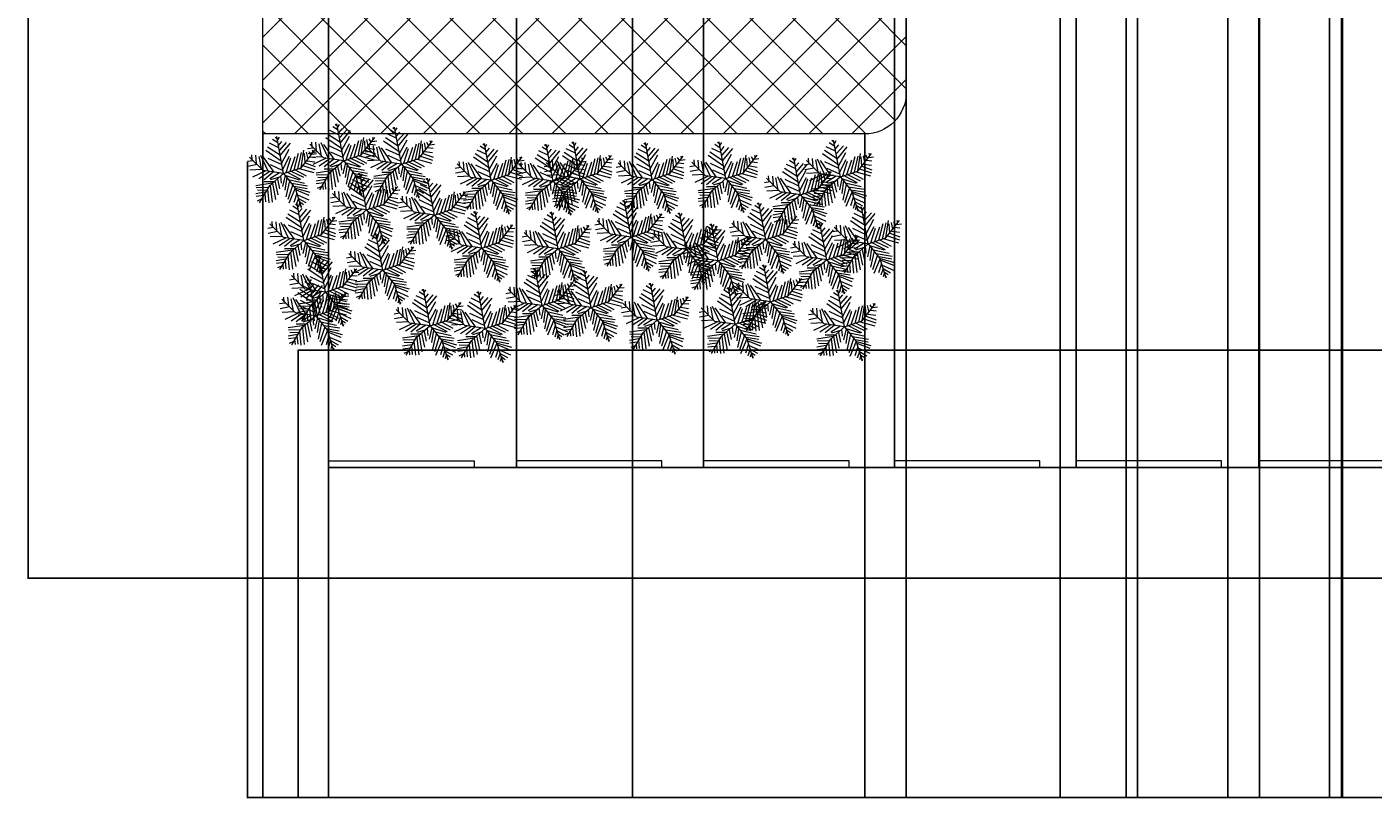
# Model space of a CAD drawing. Units: inches. Extents: x 818 to 1898, y 976 to 2364.
# Tile 1 of 96: x 818 to 1207, y 976 to 1198. Entities that reach past the tile are written whole.
import ezdxf

# ---------------------------------------------------------------- set-up
doc = ezdxf.new("R2010")
doc.units = ezdxf.units.IN
doc.header["$LTSCALE"] = 5
doc.header["$MEASUREMENT"] = 0
for name, color, linetype, lineweight in [('A-ANNO-DIMS', 2, 'Continuous', 18), ('C-PAVE-PATT', 8, 'Continuous', 9), ('C-ROAD', 8, 'Continuous', 25), ('C-ROAD-MRKG', 7, 'Continuous', 13), ('L-PAVE', 8, 'Continuous', 18)]:
    doc.layers.add(name, color=color, linetype=linetype, lineweight=lineweight)
doc.layers.add('L-PLNT', color=116, linetype='Continuous', lineweight=13, true_color=0x136734)
doc.styles.get("Standard").update_dxf_attribs({"font": 'arial.ttf'})
doc.dimstyles.get("Standard").update_dxf_attribs({"dimtxt": 0.18, "dimasz": 0.18, "dimexe": 0.18, "dimexo": 0.0625, "dimgap": 0.09, "dimtad": 0, "dimtih": 1, "dimtoh": 1, "dimdec": 4, "dimzin": 0, "dimdsep": 46, "dimtxsty": 'Standard', "dimcen": 0.09, "dimadec": 0, "dimazin": 0, "dimtfac": 1, "dimtdec": 4, "dimtofl": 0, "dimtmove": 0, "dimatfit": 3, "dimfxl": 1, "dimtolj": 1, "dimtzin": 0, "dimarcsym": 0})

# ---------------------------------------------------------------- blocks, each defined once
blk = doc.blocks.new('SHRUB-ACCENT')
for p, q in [((8.8, 18.63), (7.25, 19.67)), ((8.53, 19.84), (7.99, 20.28)), ((10.44, 9.82), (8.47, 20.47)), ((8.74, 19.5), (9.21, 20.28)), ((9.75, 13.42), (5.28, 16.46)), ((9.48, 15.07), (5.82, 17.41)), ((9.08, 17.24), (6.37, 18.54)), ((9.01, 17.93), (9.96, 19.06)), ((9.35, 16.54), (11.31, 18.8)), ((9.48, 14.98), (12.39, 18.54)), ((9.89, 12.9), (12.06, 16.89)), ((13.48, 10.9), (14.76, 15.68)), ((14.56, 11.16), (15.58, 15.85)), ((15.49, 11.5), (19.41, 16.55)), ((15.51, 11.51), (16.25, 16.54)), ((16.39, 15.59), (16.53, 12.9)), ((17, 15.94), (17.41, 14.03)), ((17.68, 16.2), (18.29, 15.16)), ((18.62, 15.42), (19.98, 15.59)), ((18.69, 16.63), (18.9, 15.94)), ((1.56, 13.51), (0, 13.25)), ((2.84, 12.38), (0.14, 11.86)), ((4.55, 10.66), (0.62, 14.58)), ((1.35, 13.77), (1.22, 15.24)), ((2.3, 15.16), (2.51, 12.72)), ((3.25, 14.72), (3.93, 11.25)), ((3.79, 15.07), (5.89, 10.55)), ((7.72, 10.21), (4.67, 14.55)), ((5.89, 14.29), (9.89, 12.38)), ((6.57, 12.38), (10.23, 10.73)), ((10.23, 11.07), (12.12, 14.81)), ((11.17, 10.12), (12.53, 14.37)), ((12.33, 10.47), (13.75, 14.72)), ((15.98, 12.12), (19.44, 10.99)), ((16.66, 12.9), (19.57, 11.86)), ((17.2, 13.51), (19.44, 13.16)), ((18.02, 14.63), (19.57, 14.46)), ((4.2, 10.99), (0.68, 10.81)), ((5.15, 10.47), (1.49, 8.73)), ((6.43, 10.38), (3.32, 8.3)), ((10.44, 9.82), (4.55, 10.66)), ((7.45, 10.21), (4.81, 8.04)), ((10.44, 9.82), (6.23, 6.17)), ((9.21, 10.03), (6.43, 8.3)), ((9.21, 8.73), (6.7, 7.95)), ((8.67, 8.21), (9.28, 5.43)), ((9.55, 9.16), (9.75, 7.08)), ((10.9, 9.25), (10.16, 6.04)), ((10.44, 9.82), (15.49, 11.5)), ((10.44, 9.82), (13.8, 5.61)), ((10.77, 9.34), (14.97, 8.04)), ((11.38, 8.64), (10.84, 5)), ((11.65, 10.12), (15.31, 8.21)), ((11.85, 8.12), (16.46, 7.08)), ((12.53, 10.47), (16.19, 8.73)), ((13.82, 10.9), (17, 9.16)), ((14.97, 11.25), (19.17, 10.12)), ((7.18, 6.99), (2.44, 6.3)), ((5.15, 4.39), (2.44, 3.95)), ((5.89, 5.78), (2.51, 5.69)), ((5.42, 4.91), (2.91, 5)), ((6.23, 6.17), (3.43, 1.4)), ((7.59, 7.43), (4.81, 7.43)), ((5.01, 4.04), (5.21, 1.61)), ((5.76, 5.34), (6.16, 1.35)), ((6.57, 6.39), (7.11, 1.52)), ((7.25, 6.99), (8.06, 2.31)), ((7.92, 7.69), (8.8, 3.69)), ((12.12, 7.69), (11.11, 3.09)), ((13.07, 6.65), (11.65, 2.31)), ((13.82, 5.6), (11.99, 1.26)), ((12.73, 6.99), (17.34, 6.3)), ((14.22, 4.13), (13.41, 1.44)), ((13.48, 6.13), (17.2, 5.52)), ((13.8, 5.61), (15.49, 0)), ((13.88, 5.6), (18.02, 4.39)), ((14.02, 5.08), (17.68, 3.61)), ((4.67, 3.43), (2.51, 3.17)), ((4, 2.39), (2.78, 1.87)), ((4.33, 2.91), (4.47, 1.52)), ((14.7, 2.74), (14.09, 0.74)), ((14.43, 3.69), (17.74, 2.22)), ((14.7, 2.65), (16.86, 1.44)), ((15.04, 1.26), (14.76, 0.31)), ((15.04, 1.7), (16.19, 0.92)), ((15.44, 0.48), (15.71, 0.31))]:
    blk.add_line(p, q)
blk = doc.blocks.new('LANE-STRIPE')
at = {"ltscale": 5}
for p, q in [((0, 2), (42, 2)), ((0, 2), (0, 0)), ((0, 0), (42, 0)), ((42, 2), (42, 0))]:
    blk.add_line(p, q, dxfattribs=at)
blk = doc.blocks.new('*D56')
at = {"layer": 'A-ANNO-DIMS', "color": 0, "lineweight": -2, "ltscale": 5, "transparency": 16777216}
for p, q in [((885.95, 1167.31), (885.95, 975.66)), ((1828.91, 1167.31), (1828.91, 975.66)), ((886.13, 975.84), (1357.14, 975.84)), ((1828.73, 975.84), (1357.72, 975.84))]:
    blk.add_line(p, q, dxfattribs=at)
at = {"layer": 'A-ANNO-DIMS', "color": 0, "ltscale": 5, "transparency": 16777216}
for points in [[(886.13, 975.87), (886.13, 975.81), (885.95, 975.84)], [(1828.73, 975.87), (1828.73, 975.81), (1828.91, 975.84)]]:
    blk.add_solid(points, dxfattribs=at)
at = {"layer": 'Defpoints', "color": 0, "ltscale": 5, "transparency": 16777216}
for p in [(885.95, 1167.37), (1828.91, 1167.37), (1828.91, 975.84)]:
    blk.add_point(p, dxfattribs=at)
at = {"layer": 'A-ANNO-DIMS', "color": 0, "ltscale": 5, "transparency": 16777216, "insert": (1357.43, 975.84), "char_height": 0.18, "attachment_point": 5}
blk.add_mtext('\\A1;943', dxfattribs=at)
blk = doc.blocks.new('*D58')
at = {"layer": 'A-ANNO-DIMS', "color": 0, "lineweight": -2, "ltscale": 5, "transparency": 16777216}
for p, q in [((881.51, 1159.31), (881.51, 975.66)), ((1834.44, 1145.13), (1834.44, 975.66)), ((881.69, 975.84), (1357.68, 975.84)), ((1834.26, 975.84), (1358.26, 975.84))]:
    blk.add_line(p, q, dxfattribs=at)
at = {"layer": 'A-ANNO-DIMS', "color": 0, "ltscale": 5, "transparency": 16777216}
for points in [[(881.69, 975.87), (881.69, 975.81), (881.51, 975.84)], [(1834.26, 975.87), (1834.26, 975.81), (1834.44, 975.84)]]:
    blk.add_solid(points, dxfattribs=at)
at = {"layer": 'Defpoints', "color": 0, "ltscale": 5, "transparency": 16777216}
for p in [(881.51, 1159.38), (1834.44, 1145.19), (1834.44, 975.84)]:
    blk.add_point(p, dxfattribs=at)
at = {"layer": 'A-ANNO-DIMS', "color": 0, "ltscale": 5, "transparency": 16777216, "insert": (1357.97, 975.84), "char_height": 0.18, "attachment_point": 5}
blk.add_mtext('\\A1;953', dxfattribs=at)
blk = doc.blocks.new('*D59')
at = {"layer": 'A-ANNO-DIMS', "color": 0, "lineweight": -2, "ltscale": 5, "transparency": 16777216}
for p, q in [((1251.64, 2300.39), (818.03, 2300.39)), ((818.21, 2300.21), (818.21, 1669.95)), ((818.21, 1039.32), (818.21, 1669.59)), ((896.05, 1039.14), (818.03, 1039.14))]:
    blk.add_line(p, q, dxfattribs=at)
at = {"layer": 'A-ANNO-DIMS', "color": 0, "ltscale": 5, "transparency": 16777216}
for points in [[(818.18, 2300.21), (818.24, 2300.21), (818.21, 2300.39)], [(818.18, 1039.32), (818.24, 1039.32), (818.21, 1039.14)]]:
    blk.add_solid(points, dxfattribs=at)
at = {"layer": 'Defpoints', "color": 0, "ltscale": 5, "transparency": 16777216}
for p in [(818.21, 2300.39), (1251.71, 2300.39), (896.11, 1039.14)]:
    blk.add_point(p, dxfattribs=at)
at = {"layer": 'A-ANNO-DIMS', "color": 0, "ltscale": 5, "transparency": 16777216, "insert": (818.21, 1669.77), "char_height": 0.18, "attachment_point": 5}
blk.add_mtext('\\A1;1261.2', dxfattribs=at)
blk = doc.blocks.new('*D62')
at = {"layer": 'A-ANNO-DIMS', "color": 0, "lineweight": -2, "ltscale": 5, "transparency": 16777216}
for p, q in [((1116.19, 1235.9), (1116.19, 975.66)), ((1406.73, 1235.9), (1406.73, 975.66)), ((1116.37, 975.84), (1260.99, 975.84)), ((1406.55, 975.84), (1261.92, 975.84))]:
    blk.add_line(p, q, dxfattribs=at)
at = {"layer": 'A-ANNO-DIMS', "color": 0, "ltscale": 5, "transparency": 16777216}
for points in [[(1116.37, 975.87), (1116.37, 975.81), (1116.19, 975.84)], [(1406.55, 975.87), (1406.55, 975.81), (1406.73, 975.84)]]:
    blk.add_solid(points, dxfattribs=at)
at = {"layer": 'Defpoints', "color": 0, "ltscale": 5, "transparency": 16777216}
for p in [(1116.19, 1235.96), (1406.73, 1235.96), (1406.73, 975.84)]:
    blk.add_point(p, dxfattribs=at)
at = {"layer": 'A-ANNO-DIMS', "color": 0, "ltscale": 5, "transparency": 16777216, "insert": (1261.46, 975.84), "char_height": 0.18, "attachment_point": 5}
blk.add_mtext('\\A1;290.54', dxfattribs=at)
blk = doc.blocks.new('*D77')
at = {"layer": 'A-ANNO-DIMS', "color": 0, "lineweight": -2, "ltscale": 5, "transparency": 16777216}
for p, q in [((992.73, 1202.9), (992.73, 975.66)), ((896.11, 1104.9), (896.11, 975.66)), ((896.29, 975.84), (944.04, 975.84)), ((992.55, 975.84), (944.8, 975.84))]:
    blk.add_line(p, q, dxfattribs=at)
at = {"layer": 'A-ANNO-DIMS', "color": 0, "ltscale": 5, "transparency": 16777216}
for points in [[(896.29, 975.87), (896.29, 975.81), (896.11, 975.84)], [(992.55, 975.87), (992.55, 975.81), (992.73, 975.84)]]:
    blk.add_solid(points, dxfattribs=at)
at = {"layer": 'Defpoints', "color": 0, "ltscale": 5, "transparency": 16777216}
for p in [(992.73, 1202.96), (896.11, 1104.97), (992.73, 975.84)]:
    blk.add_point(p, dxfattribs=at)
at = {"layer": 'A-ANNO-DIMS', "color": 0, "ltscale": 5, "transparency": 16777216, "insert": (944.42, 975.84), "char_height": 0.18, "attachment_point": 5}
blk.add_mtext('\\A1;96.61', dxfattribs=at)
blk = doc.blocks.new('*D80')
at = {"layer": 'A-ANNO-DIMS', "color": 0, "lineweight": -2, "ltscale": 5, "transparency": 16777216}
for p, q in [((1116.19, 1235.9), (1116.19, 975.66)), ((1071.73, 1202.9), (1071.73, 975.66)), ((1071.91, 975.84), (1093.56, 975.84)), ((1116.01, 975.84), (1094.35, 975.84))]:
    blk.add_line(p, q, dxfattribs=at)
at = {"layer": 'A-ANNO-DIMS', "color": 0, "ltscale": 5, "transparency": 16777216}
for points in [[(1071.91, 975.87), (1071.91, 975.81), (1071.73, 975.84)], [(1116.01, 975.87), (1116.01, 975.81), (1116.19, 975.84)]]:
    blk.add_solid(points, dxfattribs=at)
at = {"layer": 'Defpoints', "color": 0, "ltscale": 5, "transparency": 16777216}
for p in [(1116.19, 1235.96), (1071.73, 1202.96), (1116.19, 975.84)]:
    blk.add_point(p, dxfattribs=at)
at = {"layer": 'A-ANNO-DIMS', "color": 0, "ltscale": 5, "transparency": 16777216, "insert": (1093.96, 975.84), "char_height": 0.18, "attachment_point": 5}
blk.add_mtext('\\A1;44.46', dxfattribs=at)
blk = doc.blocks.new('*D88')
at = {"layer": 'A-ANNO-DIMS', "color": 0, "lineweight": -2, "ltscale": 5, "transparency": 16777216}
for p, q in [((904.95, 1070.99), (904.95, 975.66)), ((896.11, 1039.08), (896.11, 975.66)), ((896.29, 975.84), (900.14, 975.84)), ((904.77, 975.84), (900.93, 975.84))]:
    blk.add_line(p, q, dxfattribs=at)
at = {"layer": 'A-ANNO-DIMS', "color": 0, "ltscale": 5, "transparency": 16777216}
for points in [[(896.29, 975.87), (896.29, 975.81), (896.11, 975.84)], [(904.77, 975.87), (904.77, 975.81), (904.95, 975.84)]]:
    blk.add_solid(points, dxfattribs=at)
at = {"layer": 'Defpoints', "color": 0, "ltscale": 5, "transparency": 16777216}
for p in [(904.95, 1071.06), (896.11, 1039.14), (904.95, 975.84)]:
    blk.add_point(p, dxfattribs=at)
at = {"layer": 'A-ANNO-DIMS', "color": 0, "ltscale": 5, "transparency": 16777216, "insert": (900.53, 975.84), "char_height": 0.18, "attachment_point": 5}
blk.add_mtext('\\A1;8.837', dxfattribs=at)
blk = doc.blocks.new('*D89')
at = {"layer": 'A-ANNO-DIMS', "color": 0, "lineweight": -2, "ltscale": 5, "transparency": 16777216}
for p, q in [((905.01, 1071.06), (1897.92, 1071.06)), ((1897.74, 1070.88), (1897.74, 1055.28)), ((1897.74, 1039.32), (1897.74, 1054.92)), ((896.18, 1039.14), (1897.92, 1039.14))]:
    blk.add_line(p, q, dxfattribs=at)
at = {"layer": 'A-ANNO-DIMS', "color": 0, "ltscale": 5, "transparency": 16777216}
for points in [[(1897.71, 1070.88), (1897.77, 1070.88), (1897.74, 1071.06)], [(1897.71, 1039.32), (1897.77, 1039.32), (1897.74, 1039.14)]]:
    blk.add_solid(points, dxfattribs=at)
at = {"layer": 'Defpoints', "color": 0, "ltscale": 5, "transparency": 16777216}
for p in [(904.95, 1071.06), (1897.74, 1071.06), (896.11, 1039.14)]:
    blk.add_point(p, dxfattribs=at)
at = {"layer": 'A-ANNO-DIMS', "color": 0, "ltscale": 5, "transparency": 16777216, "insert": (1897.74, 1055.1), "char_height": 0.18, "attachment_point": 5}
blk.add_mtext('\\A1;31.91', dxfattribs=at)
blk = doc.blocks.new('*D90')
at = {"layer": 'A-ANNO-DIMS', "color": 0, "lineweight": -2, "ltscale": 5, "transparency": 16777216}
for p, q in [((904.95, 1071.12), (904.95, 2363.87)), ((905.13, 2363.69), (931.67, 2363.69)), ((958.99, 2363.69), (932.45, 2363.69)), ((959.17, 1071.12), (959.17, 2363.87))]:
    blk.add_line(p, q, dxfattribs=at)
at = {"layer": 'A-ANNO-DIMS', "color": 0, "ltscale": 5, "transparency": 16777216}
for points in [[(905.13, 2363.72), (905.13, 2363.66), (904.95, 2363.69)], [(958.99, 2363.72), (958.99, 2363.66), (959.17, 2363.69)]]:
    blk.add_solid(points, dxfattribs=at)
at = {"layer": 'Defpoints', "color": 0, "ltscale": 5, "transparency": 16777216}
for p in [(959.17, 2363.69), (904.95, 1071.06), (959.17, 1071.06)]:
    blk.add_point(p, dxfattribs=at)
at = {"layer": 'A-ANNO-DIMS', "color": 0, "ltscale": 5, "transparency": 16777216, "insert": (932.06, 2363.69), "char_height": 0.18, "attachment_point": 5}
blk.add_mtext('\\A1;54.22', dxfattribs=at)
blk = doc.blocks.new('*D91')
at = {"layer": 'A-ANNO-DIMS', "color": 0, "lineweight": -2, "ltscale": 5, "transparency": 16777216}
for p, q in [((959.17, 1071.12), (959.17, 2363.87)), ((959.35, 2363.69), (985.8, 2363.69)), ((1013.04, 2363.69), (986.59, 2363.69)), ((1013.22, 1071.12), (1013.22, 2363.87))]:
    blk.add_line(p, q, dxfattribs=at)
at = {"layer": 'A-ANNO-DIMS', "color": 0, "ltscale": 5, "transparency": 16777216}
for points in [[(959.35, 2363.72), (959.35, 2363.66), (959.17, 2363.69)], [(1013.04, 2363.72), (1013.04, 2363.66), (1013.22, 2363.69)]]:
    blk.add_solid(points, dxfattribs=at)
at = {"layer": 'Defpoints', "color": 0, "ltscale": 5, "transparency": 16777216}
for p in [(1013.22, 2363.69), (959.17, 1071.06), (1013.22, 1071.06)]:
    blk.add_point(p, dxfattribs=at)
at = {"layer": 'A-ANNO-DIMS', "color": 0, "ltscale": 5, "transparency": 16777216, "insert": (986.2, 2363.69), "char_height": 0.18, "attachment_point": 5}
blk.add_mtext('\\A1;54.04', dxfattribs=at)
blk = doc.blocks.new('*D92')
at = {"layer": 'A-ANNO-DIMS', "color": 0, "lineweight": -2, "ltscale": 5, "transparency": 16777216}
for p, q in [((1013.22, 1071.12), (1013.22, 2363.87)), ((1013.4, 2363.69), (1040.38, 2363.69)), ((1068.16, 2363.69), (1041.17, 2363.69)), ((1068.34, 1071.12), (1068.34, 2363.87))]:
    blk.add_line(p, q, dxfattribs=at)
at = {"layer": 'A-ANNO-DIMS', "color": 0, "ltscale": 5, "transparency": 16777216}
for points in [[(1013.4, 2363.72), (1013.4, 2363.66), (1013.22, 2363.69)], [(1068.16, 2363.72), (1068.16, 2363.66), (1068.34, 2363.69)]]:
    blk.add_solid(points, dxfattribs=at)
at = {"layer": 'Defpoints', "color": 0, "ltscale": 5, "transparency": 16777216}
for p in [(1068.34, 2363.69), (1013.22, 1071.06), (1068.34, 1071.06)]:
    blk.add_point(p, dxfattribs=at)
at = {"layer": 'A-ANNO-DIMS', "color": 0, "ltscale": 5, "transparency": 16777216, "insert": (1040.78, 2363.69), "char_height": 0.18, "attachment_point": 5}
blk.add_mtext('\\A1;55.12', dxfattribs=at)
blk = doc.blocks.new('*D93')
at = {"layer": 'A-ANNO-DIMS', "color": 0, "lineweight": -2, "ltscale": 5, "transparency": 16777216}
for p, q in [((1068.34, 1071.12), (1068.34, 2363.87)), ((1068.52, 2363.69), (1094.16, 2363.69)), ((1120.58, 2363.69), (1094.94, 2363.69)), ((1120.76, 1071.12), (1120.76, 2363.87))]:
    blk.add_line(p, q, dxfattribs=at)
at = {"layer": 'A-ANNO-DIMS', "color": 0, "ltscale": 5, "transparency": 16777216}
for points in [[(1068.52, 2363.72), (1068.52, 2363.66), (1068.34, 2363.69)], [(1120.58, 2363.72), (1120.58, 2363.66), (1120.76, 2363.69)]]:
    blk.add_solid(points, dxfattribs=at)
at = {"layer": 'Defpoints', "color": 0, "ltscale": 5, "transparency": 16777216}
for p in [(1120.76, 2363.69), (1068.34, 1071.06), (1120.76, 1071.06)]:
    blk.add_point(p, dxfattribs=at)
at = {"layer": 'A-ANNO-DIMS', "color": 0, "ltscale": 5, "transparency": 16777216, "insert": (1094.55, 2363.69), "char_height": 0.18, "attachment_point": 5}
blk.add_mtext('\\A1;52.42', dxfattribs=at)
blk = doc.blocks.new('*D94')
at = {"layer": 'A-ANNO-DIMS', "color": 0, "lineweight": -2, "ltscale": 5, "transparency": 16777216}
for p, q in [((1120.76, 1071.12), (1120.76, 2363.87)), ((1120.94, 2363.69), (1146.76, 2363.69)), ((1173.36, 2363.69), (1147.55, 2363.69)), ((1173.54, 1071.12), (1173.54, 2363.87))]:
    blk.add_line(p, q, dxfattribs=at)
at = {"layer": 'A-ANNO-DIMS', "color": 0, "ltscale": 5, "transparency": 16777216}
for points in [[(1120.94, 2363.72), (1120.94, 2363.66), (1120.76, 2363.69)], [(1173.36, 2363.72), (1173.36, 2363.66), (1173.54, 2363.69)]]:
    blk.add_solid(points, dxfattribs=at)
at = {"layer": 'Defpoints', "color": 0, "ltscale": 5, "transparency": 16777216}
for p in [(1173.54, 2363.69), (1120.76, 1071.06), (1173.54, 1071.06)]:
    blk.add_point(p, dxfattribs=at)
at = {"layer": 'A-ANNO-DIMS', "color": 0, "ltscale": 5, "transparency": 16777216, "insert": (1147.15, 2363.69), "char_height": 0.18, "attachment_point": 5}
blk.add_mtext('\\A1;52.78', dxfattribs=at)
blk = doc.blocks.new('*D95')
at = {"layer": 'A-ANNO-DIMS', "color": 0, "lineweight": -2, "ltscale": 5, "transparency": 16777216}
for p, q in [((1173.54, 1071.12), (1173.54, 2363.87)), ((1173.72, 2363.69), (1201.29, 2363.69)), ((1229.47, 2363.69), (1201.9, 2363.69)), ((1229.65, 1071.12), (1229.65, 2363.87))]:
    blk.add_line(p, q, dxfattribs=at)
at = {"layer": 'A-ANNO-DIMS', "color": 0, "ltscale": 5, "transparency": 16777216}
for points in [[(1173.72, 2363.72), (1173.72, 2363.66), (1173.54, 2363.69)], [(1229.47, 2363.72), (1229.47, 2363.66), (1229.65, 2363.69)]]:
    blk.add_solid(points, dxfattribs=at)
at = {"layer": 'Defpoints', "color": 0, "ltscale": 5, "transparency": 16777216}
for p in [(1229.65, 2363.69), (1173.54, 1071.06), (1229.65, 1071.06)]:
    blk.add_point(p, dxfattribs=at)
at = {"layer": 'A-ANNO-DIMS', "color": 0, "ltscale": 5, "transparency": 16777216, "insert": (1201.59, 2363.69), "char_height": 0.18, "attachment_point": 5}
blk.add_mtext('\\A1;56.1', dxfattribs=at)
blk = doc.blocks.new('*D105')
at = {"layer": 'A-ANNO-DIMS', "color": 0, "lineweight": -2, "ltscale": 5, "transparency": 16777216}
for p, q in [((1164.56, 1248.4), (1164.56, 975.66)), ((1116.19, 1235.9), (1116.19, 975.66)), ((1116.37, 975.84), (1139.98, 975.84)), ((1164.38, 975.84), (1140.77, 975.84))]:
    blk.add_line(p, q, dxfattribs=at)
at = {"layer": 'A-ANNO-DIMS', "color": 0, "ltscale": 5, "transparency": 16777216}
for points in [[(1116.37, 975.87), (1116.37, 975.81), (1116.19, 975.84)], [(1164.38, 975.87), (1164.38, 975.81), (1164.56, 975.84)]]:
    blk.add_solid(points, dxfattribs=at)
at = {"layer": 'Defpoints', "color": 0, "ltscale": 5, "transparency": 16777216}
for p in [(1164.56, 1248.46), (1116.19, 1235.96), (1164.56, 975.84)]:
    blk.add_point(p, dxfattribs=at)
at = {"layer": 'A-ANNO-DIMS', "color": 0, "ltscale": 5, "transparency": 16777216, "insert": (1140.37, 975.84), "char_height": 0.18, "attachment_point": 5}
blk.add_mtext('\\A1;48.37', dxfattribs=at)
blk = doc.blocks.new('*D106')
at = {"layer": 'A-ANNO-DIMS', "color": 0, "lineweight": -2, "ltscale": 5, "transparency": 16777216}
for p, q in [((1164.56, 1248.4), (1164.56, 975.66)), ((1252.11, 1248.4), (1252.11, 975.66)), ((1164.74, 975.84), (1207.94, 975.84)), ((1251.93, 975.84), (1208.73, 975.84))]:
    blk.add_line(p, q, dxfattribs=at)
at = {"layer": 'A-ANNO-DIMS', "color": 0, "ltscale": 5, "transparency": 16777216}
for points in [[(1164.74, 975.87), (1164.74, 975.81), (1164.56, 975.84)], [(1251.93, 975.87), (1251.93, 975.81), (1252.11, 975.84)]]:
    blk.add_solid(points, dxfattribs=at)
at = {"layer": 'Defpoints', "color": 0, "ltscale": 5, "transparency": 16777216}
for p in [(1164.56, 1248.46), (1252.11, 1248.46), (1252.11, 975.84)]:
    blk.add_point(p, dxfattribs=at)
at = {"layer": 'A-ANNO-DIMS', "color": 0, "ltscale": 5, "transparency": 16777216, "insert": (1208.33, 975.84), "char_height": 0.18, "attachment_point": 5}
blk.add_mtext('\\A1;87.55', dxfattribs=at)
blk = doc.blocks.new('*D111')
at = {"layer": 'A-ANNO-DIMS', "color": 0, "lineweight": -2, "ltscale": 5, "transparency": 16777216}
for p, q in [((1135.21, 1405.65), (1135.21, 975.66)), ((1193.91, 1405.65), (1193.91, 975.66)), ((1135.39, 975.84), (1164.23, 975.84)), ((1193.73, 975.84), (1164.88, 975.84))]:
    blk.add_line(p, q, dxfattribs=at)
at = {"layer": 'A-ANNO-DIMS', "color": 0, "ltscale": 5, "transparency": 16777216}
for points in [[(1135.39, 975.87), (1135.39, 975.81), (1135.21, 975.84)], [(1193.73, 975.87), (1193.73, 975.81), (1193.91, 975.84)]]:
    blk.add_solid(points, dxfattribs=at)
at = {"layer": 'Defpoints', "color": 0, "ltscale": 5, "transparency": 16777216}
for p in [(1135.21, 1405.71), (1193.91, 1405.71), (1193.91, 975.84)]:
    blk.add_point(p, dxfattribs=at)
at = {"layer": 'A-ANNO-DIMS', "color": 0, "ltscale": 5, "transparency": 16777216, "insert": (1164.56, 975.84), "char_height": 0.18, "attachment_point": 5}
blk.add_mtext('\\A1;58.7', dxfattribs=at)
blk = doc.blocks.new('*D122')
at = {"layer": 'A-ANNO-DIMS', "color": 0, "lineweight": -2, "ltscale": 5, "transparency": 16777216}
for p, q in [((1138.5, 1794.37), (1138.5, 975.66)), ((1071.73, 1688.02), (1071.73, 975.66)), ((1071.91, 975.84), (1104.72, 975.84)), ((1138.32, 975.84), (1105.51, 975.84))]:
    blk.add_line(p, q, dxfattribs=at)
at = {"layer": 'A-ANNO-DIMS', "color": 0, "ltscale": 5, "transparency": 16777216}
for points in [[(1071.91, 975.87), (1071.91, 975.81), (1071.73, 975.84)], [(1138.32, 975.87), (1138.32, 975.81), (1138.5, 975.84)]]:
    blk.add_solid(points, dxfattribs=at)
at = {"layer": 'Defpoints', "color": 0, "ltscale": 5, "transparency": 16777216}
for p in [(1138.5, 1794.43), (1071.73, 1688.08), (1138.5, 975.84)]:
    blk.add_point(p, dxfattribs=at)
at = {"layer": 'A-ANNO-DIMS', "color": 0, "ltscale": 5, "transparency": 16777216, "insert": (1105.11, 975.84), "char_height": 0.18, "attachment_point": 5}
blk.add_mtext('\\A1;66.78', dxfattribs=at)
blk = doc.blocks.new('*D145')
at = {"layer": 'A-ANNO-DIMS', "color": 0, "lineweight": -2, "ltscale": 5, "transparency": 16777216}
for p, q in [((1197.39, 2122.31), (1197.39, 975.66)), ((1232.61, 2122.31), (1232.61, 975.66)), ((1197.57, 975.84), (1214.61, 975.84)), ((1232.43, 975.84), (1215.39, 975.84))]:
    blk.add_line(p, q, dxfattribs=at)
at = {"layer": 'A-ANNO-DIMS', "color": 0, "ltscale": 5, "transparency": 16777216}
for points in [[(1197.57, 975.87), (1197.57, 975.81), (1197.39, 975.84)], [(1232.43, 975.87), (1232.43, 975.81), (1232.61, 975.84)]]:
    blk.add_solid(points, dxfattribs=at)
at = {"layer": 'Defpoints', "color": 0, "ltscale": 5, "transparency": 16777216}
for p in [(1197.39, 2122.38), (1232.61, 2122.38), (1232.61, 975.84)]:
    blk.add_point(p, dxfattribs=at)
at = {"layer": 'A-ANNO-DIMS', "color": 0, "ltscale": 5, "transparency": 16777216, "insert": (1215, 975.84), "char_height": 0.18, "attachment_point": 5}
blk.add_mtext('\\A1;35.22', dxfattribs=at)
blk = doc.blocks.new('*D151')
at = {"layer": 'A-ANNO-DIMS', "color": 0, "lineweight": -2, "ltscale": 5, "transparency": 16777216}
for p, q in [((1071.73, 1179.31), (1071.73, 975.66)), ((1059.73, 1167.31), (1059.73, 975.66)), ((1059.91, 975.84), (1065.52, 975.84)), ((1071.55, 975.84), (1065.93, 975.84))]:
    blk.add_line(p, q, dxfattribs=at)
at = {"layer": 'A-ANNO-DIMS', "color": 0, "ltscale": 5, "transparency": 16777216}
for points in [[(1059.91, 975.87), (1059.91, 975.81), (1059.73, 975.84)], [(1071.55, 975.87), (1071.55, 975.81), (1071.73, 975.84)]]:
    blk.add_solid(points, dxfattribs=at)
at = {"layer": 'Defpoints', "color": 0, "ltscale": 5, "transparency": 16777216}
for p in [(1071.73, 1179.37), (1059.73, 1167.37), (1059.73, 975.84)]:
    blk.add_point(p, dxfattribs=at)
at = {"layer": 'A-ANNO-DIMS', "color": 0, "ltscale": 5, "transparency": 16777216, "insert": (1065.73, 975.84), "char_height": 0.18, "attachment_point": 5}
blk.add_mtext('\\A1;12', dxfattribs=at)
blk = doc.blocks.new('*D155')
at = {"layer": 'A-ANNO-DIMS', "color": 0, "lineweight": -2, "ltscale": 5, "transparency": 16777216}
for p, q in [((1173.73, 1590.7), (1173.73, 975.66)), ((1197.73, 1530.54), (1197.73, 975.66)), ((1173.91, 975.84), (1185.51, 975.84)), ((1197.55, 975.84), (1185.95, 975.84))]:
    blk.add_line(p, q, dxfattribs=at)
at = {"layer": 'A-ANNO-DIMS', "color": 0, "ltscale": 5, "transparency": 16777216}
for points in [[(1173.91, 975.87), (1173.91, 975.81), (1173.73, 975.84)], [(1197.55, 975.87), (1197.55, 975.81), (1197.73, 975.84)]]:
    blk.add_solid(points, dxfattribs=at)
at = {"layer": 'Defpoints', "color": 0, "ltscale": 5, "transparency": 16777216}
for p in [(1173.73, 1590.76), (1197.73, 1530.6), (1173.73, 975.84)]:
    blk.add_point(p, dxfattribs=at)
at = {"layer": 'A-ANNO-DIMS', "color": 0, "ltscale": 5, "transparency": 16777216, "insert": (1185.73, 975.84), "char_height": 0.18, "attachment_point": 5}
blk.add_mtext('\\A1;24', dxfattribs=at)

msp = doc.modelspace()

# ---------------------------------------------------------------- hatches: boundary and pattern name
at = {"layer": 'C-PAVE-PATT', "ltscale": 5}
h = msp.add_hatch(dxfattribs=at)
h.set_pattern_fill('ANSI37', color=256, scale=70)
h.paths.add_polyline_path([(1071.7251, 1202.9642), (885.9457, 1202.9642), (885.9457, 1167.3717), (1059.7251, 1167.3717, 0.41421356), (1071.7251, 1179.3717)])
h.paths.add_polyline_path([(1828.9123, 1202.9642), (1430.7252, 1202.9642), (1430.7252, 1179.3717, 0.41421356), (1442.7252, 1167.3717), (1828.9123, 1167.3717)])

# ---------------------------------------------------------------- linework, layer by layer
at = {"layer": 'C-ROAD', "ltscale": 5}
msp.add_lwpolyline([(1828.9123, 1104.9672), (896.1138, 1104.9672), (896.1138, 1039.1433), (1828.9123, 1039.1433)], close=True, dxfattribs=at)
at = {"layer": 'L-PAVE', "ltscale": 5}
msp.add_lwpolyline([(885.9457, 1202.9642), (1071.7251, 1202.9642), (1071.7251, 1179.3717, -0.41421356), (1059.7251, 1167.3717), (885.9457, 1167.3717)], format="xyb", close=True, dxfattribs=at)

# ---------------------------------------------------------------- block references
at = {"layer": 'C-ROAD-MRKG'}
msp.add_blockref('LANE-STRIPE', (904.95, 1071.055), dxfattribs=at)
at = {"layer": 'C-ROAD-MRKG', "rotation": 180}
for p in [(1001.1748, 1073.0554), (1055.2188, 1073.0554), (1110.3388, 1073.0554), (1162.7629, 1073.0554), (1215.543, 1073.0554)]:
    msp.add_blockref('LANE-STRIPE', p, dxfattribs=at)
at = {"layer": 'L-PLNT'}
for p in [(898.879, 1149.7974), (881.5059, 1146.13), (915.5179, 1148.8194), (941.4551, 1144.1741), (959.3175, 1143.9296), (967.1737, 1144.5808), (987.9463, 1144.4186), (1009.2344, 1144.6631), (1042.2676, 1145.152), (1030.7671, 1140.0178), (905.4856, 1135.6169), (925.0608, 1134.15), (887.3785, 1126.8153), (981.829, 1127.7932), (1020.7348, 1127.0598), (938.7635, 1124.6149), (960.7856, 1124.3704), (997.8213, 1124.16), (1050.3424, 1125.8373), (1007.0321, 1120.9475), (1038.3525, 1121.192), (910.1347, 1118.2581), (893.6487, 1111.915), (956.1365, 1107.9895), (970.3286, 1107.5006), (1022.1269, 1109.1242), (890.8042, 1105.0557), (989.4144, 1103.8332), (923.8374, 1102.1218), (939.7423, 1101.3883), (1011.926, 1102.6108), (1043.491, 1101.8773)]:
    msp.add_blockref('SHRUB-ACCENT', p, dxfattribs=at)

# ---------------------------------------------------------------- dimensions: what is measured, and where the dimension line sits
at = {"layer": 'A-ANNO-DIMS', "ltscale": 5}
for base, p1, p2, override, picture, middle in [((959.1737, 2363.6929), (904.9504, 1071.0552), (959.1737, 1071.0552), {"dimdec": 2, "dimlfac": 1, "dimrnd": 0, "dimzin": 0, "dimdsep": 46, "dimlunit": 2}, '*D90', (932.062, 2363.6929)), ((1013.2176, 2363.6929), (959.1737, 1071.0552), (1013.2176, 1071.0552), {"dimdec": 2, "dimlfac": 1, "dimrnd": 0, "dimzin": 0, "dimdsep": 46, "dimlunit": 2}, '*D91', (986.1956, 2363.6929)), ((1068.3377, 2363.6929), (1013.2176, 1071.0552), (1068.3377, 1071.0552), {"dimdec": 2, "dimlfac": 1, "dimrnd": 0, "dimzin": 0, "dimdsep": 46, "dimlunit": 2}, '*D92', (1040.7776, 2363.6929)), ((1120.7618, 2363.6929), (1068.3377, 1071.0552), (1120.7618, 1071.0552), {"dimdec": 2, "dimlfac": 1, "dimrnd": 0, "dimzin": 0, "dimdsep": 46, "dimlunit": 2}, '*D93', (1094.5497, 2363.6929)), ((1173.5418, 2363.6929), (1120.7618, 1071.0552), (1173.5418, 1071.0552), {"dimdec": 2, "dimlfac": 1, "dimrnd": 0, "dimzin": 0, "dimdsep": 46, "dimlunit": 2}, '*D94', (1147.1518, 2363.6929)), ((1229.6474, 2363.6929), (1173.5418, 1071.0552), (1229.6474, 1071.0552), {"dimdec": 1, "dimlfac": 1, "dimrnd": 0, "dimzin": 0, "dimdsep": 46, "dimlunit": 2}, '*D95', (1201.5946, 2363.6929)), ((1232.6091, 975.8433), (1197.3925, 2122.3767), (1232.6091, 2122.3767), {"dimdec": 2, "dimlfac": 1, "dimrnd": 0, "dimzin": 0, "dimdsep": 46, "dimlunit": 2}, '*D145', (1215.0008, 975.8433)), ((1138.5041, 975.8433), (1071.7251, 1688.0782), (1138.5041, 1794.4325), {"dimdec": 2, "dimlfac": 1, "dimrnd": 0, "dimzin": 0, "dimdsep": 46, "dimlunit": 2}, '*D122', (1105.1146, 975.8433)), ((1173.7251, 975.8433), (1197.7251, 1530.6024), (1173.7251, 1590.7585), {"dimdec": 0, "dimlfac": 1, "dimrnd": 0, "dimzin": 0, "dimdsep": 46, "dimlunit": 2}, '*D155', (1185.7251, 975.8433)), ((1193.9083, 975.8433), (1135.2058, 1405.7088), (1193.9083, 1405.7088), {"dimdec": 1, "dimlfac": 1, "dimrnd": 0, "dimzin": 0, "dimdsep": 46, "dimlunit": 2}, '*D111', (1164.5571, 975.8433)), ((1164.5571, 975.8433), (1116.1882, 1235.9642), (1164.5571, 1248.4622), {"dimdec": 2, "dimlfac": 1, "dimrnd": 0, "dimzin": 0, "dimdsep": 46, "dimlunit": 2}, '*D105', (1140.3726, 975.8433)), ((1252.1115, 975.8433), (1164.5571, 1248.4622), (1252.1115, 1248.4622), {"dimdec": 2, "dimlfac": 1, "dimrnd": 0, "dimzin": 0, "dimdsep": 46, "dimlunit": 2}, '*D106', (1208.3343, 975.8433)), ((1116.1882, 975.8433), (1071.7251, 1202.9642), (1116.1882, 1235.9642), {"dimdec": 2, "dimlfac": 1, "dimrnd": 0, "dimzin": 0, "dimdsep": 46, "dimlunit": 2}, '*D80', (1093.9567, 975.8433)), ((1406.7251, 975.8433), (1116.1882, 1235.9642), (1406.7251, 1235.9642), {"dimdec": 2, "dimlfac": 1, "dimrnd": 0, "dimzin": 0, "dimdsep": 46, "dimlunit": 2}, '*D62', (1261.4567, 975.8433)), ((992.7251, 975.8433), (896.1138, 1104.9672), (992.7251, 1202.9642), {"dimdec": 2, "dimlfac": 1, "dimrnd": 0, "dimzin": 0, "dimdsep": 46, "dimlunit": 2}, '*D77', (944.4195, 975.8433)), ((1059.7251, 975.8433), (1071.7251, 1179.3717), (1059.7251, 1167.3717), {"dimdec": 0, "dimlfac": 1, "dimrnd": 0, "dimzin": 0, "dimdsep": 46, "dimlunit": 2}, '*D151', (1065.7251, 975.8433)), ((1828.9123, 975.8433), (885.9457, 1167.3717), (1828.9123, 1167.3717), {"dimdec": 0, "dimlfac": 1, "dimrnd": 0, "dimzin": 0, "dimdsep": 46, "dimlunit": 2}, '*D56', (1357.429, 975.8433)), ((1834.436, 975.8433), (881.5059, 1159.375), (1834.436, 1145.1942), {"dimdec": 0, "dimlfac": 1, "dimrnd": 0, "dimzin": 0, "dimdsep": 46, "dimlunit": 2}, '*D58', (1357.971, 975.8433)), ((904.9504, 975.8433), (896.1138, 1039.1433), (904.9504, 1071.0552), {"dimdec": 3, "dimlfac": 1, "dimrnd": 0, "dimzin": 0, "dimdsep": 46, "dimlunit": 2}, '*D88', (900.5321, 975.8433))]:
    dim = msp.add_linear_dim(base=base, p1=p1, p2=p2, dimstyle='Standard', override=override, dxfattribs=at)
    dim.commit()
    dim.dimension.update_dxf_attribs({"geometry": picture, "text_midpoint": middle})
for base, p2, override, picture, middle in [((818.2059, 2300.3929), (1251.7057, 2300.3929), {"dimdec": 1, "dimlfac": 1, "dimrnd": 0, "dimzin": 0, "dimdsep": 46, "dimlunit": 2}, '*D59', (818.2059, 1669.7681)), ((1897.736, 1071.0552), (904.9504, 1071.0552), {"dimdec": 2, "dimlfac": 1, "dimrnd": 0, "dimzin": 0, "dimdsep": 46, "dimlunit": 2}, '*D89', (1897.736, 1055.0992))]:
    dim = msp.add_linear_dim(base=base, p1=(896.1138, 1039.1433), p2=p2, angle=90, dimstyle='Standard', override=override, dxfattribs=at)
    dim.commit()
    dim.dimension.update_dxf_attribs({"geometry": picture, "text_midpoint": middle})

doc.saveas('drawing.dxf')
